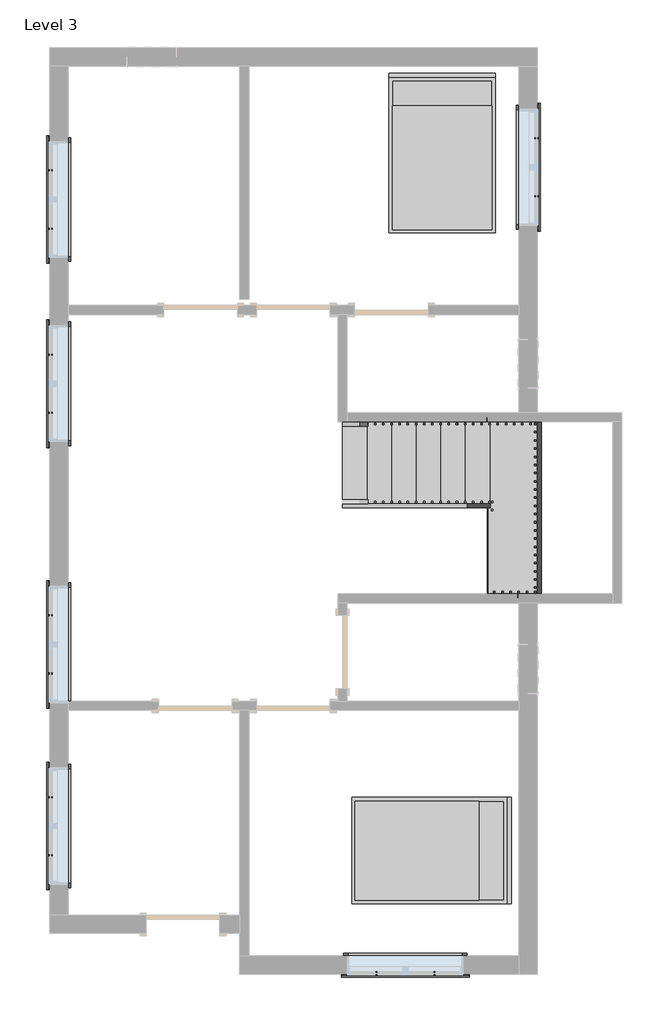
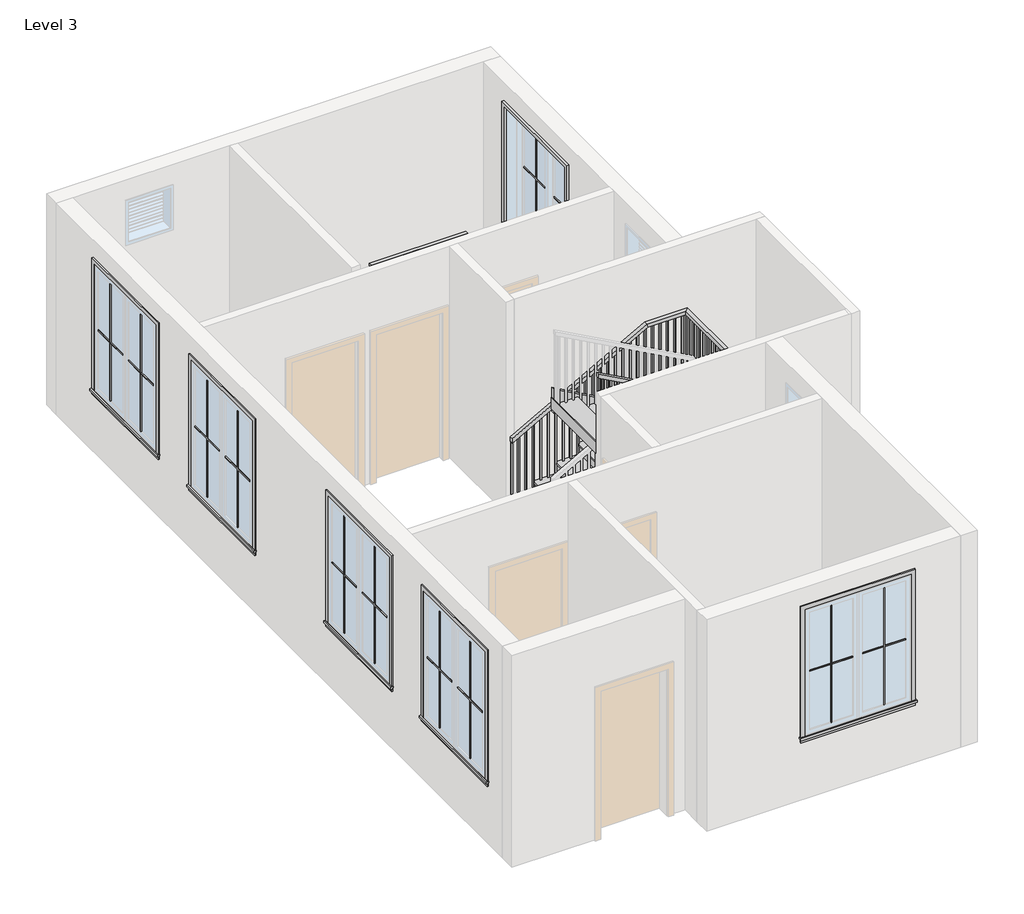
# One storey, part 2 of 2: 24 proxies, 5 members, 2 furniture elements, 1 railing, 1 stair flight.
"""IFC4 building model written with IfcOpenShell, lengths in millimetres."""

from ifc_helpers import new_model, si_unit, frame, origin, place, context, project, spatial, polyline, outline, extrude, faceted_brep, transform, mapped, element, save
from components import muntin_pattern_2x2_muntin_pattern_2x2_bff912c5, muntin_pattern_2x2_muntin_pattern_2x2_c2194282, trim_window_exterior_flat_with_sill_e04b3088, trim_window_interior_flat_picture_frame_2a7685fe, bed_17739_bed_17739_15c61121, stair_flight_656f6d92

model = new_model("IFC4")

# Units and contexts
model_context = context("Model", 3, world=origin())
ifc_project = project(units=[si_unit("LENGTHUNIT", "METRE", prefix="MILLI")], contexts=[model_context])

# Site, building, storey
site = spatial("IfcSite", under=ifc_project)
building = spatial("IfcBuilding", under=site)
storey = spatial("IfcBuildingStorey", under=building, Name="Level 3", Elevation=3200.4)

# Proxies
placement = place(None, origin())
muntin_pattern_2x2_muntin_pattern_2x2_shape = muntin_pattern_2x2_muntin_pattern_2x2_bff912c5(model_context)
element("IfcBuildingElementProxy", 1, Name="Muntin Pattern_2x2 : Muntin Pattern_2x2", ObjectType="Muntin Pattern_2x2 : Muntin Pattern_2x2", at=placement, inside=storey, context=model_context, shape_type="MappedRepresentation", body=[
    mapped(muntin_pattern_2x2_muntin_pattern_2x2_shape, transform((-4796.6888307, -4528.6107799, 4184.65), x_axis=(0.0, 1.0, 0.0), y_axis=(-1.0, 0.0, 0.0), z_axis=(0.0, 0.0, 1.0))),
])
element("IfcBuildingElementProxy", 2, Name="Muntin Pattern_2x2 : Muntin Pattern_2x2", ObjectType="Muntin Pattern_2x2 : Muntin Pattern_2x2", at=placement, inside=storey, context=model_context, shape_type="MappedRepresentation", body=[
    mapped(muntin_pattern_2x2_muntin_pattern_2x2_shape, transform((-4796.6888307, -2274.3607799, 4184.65), x_axis=(0.0, 1.0, 0.0), y_axis=(-1.0, 0.0, 0.0), z_axis=(0.0, 0.0, 1.0))),
])
element("IfcBuildingElementProxy", 3, Name="Muntin Pattern_2x2 : Muntin Pattern_2x2", ObjectType="Muntin Pattern_2x2 : Muntin Pattern_2x2", at=placement, inside=storey, context=model_context, shape_type="MappedRepresentation", body=[
    mapped(muntin_pattern_2x2_muntin_pattern_2x2_shape, transform((-26.2513307, -6000.2232799, 4184.65), x_axis=(-1.0, 0.0, 0.0), y_axis=(0.0, -1.0, 0.0), z_axis=(0.0, 0.0, 1.0))),
])
element("IfcBuildingElementProxy", 4, Name="Muntin Pattern_2x2 : Muntin Pattern_2x2", ObjectType="Muntin Pattern_2x2 : Muntin Pattern_2x2", at=placement, inside=storey, context=model_context, shape_type="MappedRepresentation", body=[
    mapped(muntin_pattern_2x2_muntin_pattern_2x2_shape, transform((1242.1611693, 4370.9142201, 4184.65), x_axis=(0.0, -1.0, 0.0), y_axis=(1.0, 0.0, 0.0), z_axis=(0.0, 0.0, 1.0))),
])
element("IfcBuildingElementProxy", 5, Name="Muntin Pattern_2x2 : Muntin Pattern_2x2", ObjectType="Muntin Pattern_2x2 : Muntin Pattern_2x2", at=placement, inside=storey, context=model_context, shape_type="MappedRepresentation", body=[
    mapped(muntin_pattern_2x2_muntin_pattern_2x2_shape, transform((-4796.6888307, 3250.1392201, 4184.65), x_axis=(0.0, 1.0, 0.0), y_axis=(-1.0, 0.0, 0.0), z_axis=(0.0, 0.0, 1.0))),
])
element("IfcBuildingElementProxy", 6, Name="Muntin Pattern_2x2 : Muntin Pattern_2x2", ObjectType="Muntin Pattern_2x2 : Muntin Pattern_2x2", at=placement, inside=storey, context=model_context, shape_type="MappedRepresentation", body=[
    mapped(muntin_pattern_2x2_muntin_pattern_2x2_shape, transform((-4796.6888307, 964.1392201, 4184.65), x_axis=(0.0, 1.0, 0.0), y_axis=(-1.0, 0.0, 0.0), z_axis=(0.0, 0.0, 1.0))),
])
muntin_pattern_2x2_muntin_pattern_2x2_2_shape = muntin_pattern_2x2_muntin_pattern_2x2_c2194282(model_context)
element("IfcBuildingElementProxy", 7, Name="Muntin Pattern_2x2 : Muntin Pattern_2x2", ObjectType="Muntin Pattern_2x2 : Muntin Pattern_2x2", at=placement, inside=storey, context=model_context, shape_type="MappedRepresentation", body=[
    mapped(muntin_pattern_2x2_muntin_pattern_2x2_2_shape, transform((-4796.6888307, -3807.8857799, 4184.65), x_axis=(0.0, -1.0, 0.0), y_axis=(1.0, 0.0, 0.0), z_axis=(0.0, 0.0, 1.0))),
])
element("IfcBuildingElementProxy", 8, Name="Muntin Pattern_2x2 : Muntin Pattern_2x2", ObjectType="Muntin Pattern_2x2 : Muntin Pattern_2x2", at=placement, inside=storey, context=model_context, shape_type="MappedRepresentation", body=[
    mapped(muntin_pattern_2x2_muntin_pattern_2x2_2_shape, transform((-4796.6888307, -1553.6357799, 4184.65), x_axis=(0.0, -1.0, 0.0), y_axis=(1.0, 0.0, 0.0), z_axis=(0.0, 0.0, 1.0))),
])
element("IfcBuildingElementProxy", 9, Name="Muntin Pattern_2x2 : Muntin Pattern_2x2", ObjectType="Muntin Pattern_2x2 : Muntin Pattern_2x2", at=placement, inside=storey, context=model_context, shape_type="MappedRepresentation", body=[
    mapped(muntin_pattern_2x2_muntin_pattern_2x2_2_shape, transform((-746.9763307, -6000.2232799, 4184.65), x_axis=(1.0, 0.0, 0.0), y_axis=(0.0, 1.0, 0.0), z_axis=(0.0, 0.0, 1.0))),
])
element("IfcBuildingElementProxy", 10, Name="Muntin Pattern_2x2 : Muntin Pattern_2x2", ObjectType="Muntin Pattern_2x2 : Muntin Pattern_2x2", at=placement, inside=storey, context=model_context, shape_type="MappedRepresentation", body=[
    mapped(muntin_pattern_2x2_muntin_pattern_2x2_2_shape, transform((1242.1611693, 3650.1892201, 4184.65), x_axis=(0.0, 1.0, 0.0), y_axis=(-1.0, 0.0, 0.0), z_axis=(0.0, 0.0, 1.0))),
])
element("IfcBuildingElementProxy", 11, Name="Muntin Pattern_2x2 : Muntin Pattern_2x2", ObjectType="Muntin Pattern_2x2 : Muntin Pattern_2x2", at=placement, inside=storey, context=model_context, shape_type="MappedRepresentation", body=[
    mapped(muntin_pattern_2x2_muntin_pattern_2x2_2_shape, transform((-4796.6888307, 3970.8642201, 4184.65), x_axis=(0.0, -1.0, 0.0), y_axis=(1.0, 0.0, 0.0), z_axis=(0.0, 0.0, 1.0))),
])
element("IfcBuildingElementProxy", 12, Name="Muntin Pattern_2x2 : Muntin Pattern_2x2", ObjectType="Muntin Pattern_2x2 : Muntin Pattern_2x2", at=placement, inside=storey, context=model_context, shape_type="MappedRepresentation", body=[
    mapped(muntin_pattern_2x2_muntin_pattern_2x2_2_shape, transform((-4796.6888307, 1684.8642201, 4184.65), x_axis=(0.0, -1.0, 0.0), y_axis=(1.0, 0.0, 0.0), z_axis=(0.0, 0.0, 1.0))),
])
trim_window_exterior_flat_with_sill_shape = trim_window_exterior_flat_with_sill_e04b3088(model_context)
element("IfcBuildingElementProxy", 13, Name="Trim-Window-Exterior-Flat : with Sill", ObjectType="Trim-Window-Exterior-Flat : with Sill", at=placement, inside=storey, context=model_context, shape_type="MappedRepresentation", body=[
    mapped(trim_window_exterior_flat_with_sill_shape, transform((-4806.2138307, -4168.2482799, 5943.6), x_axis=(0.0, -1.0, 0.0), y_axis=(0.0, 0.0, 1.0), z_axis=(-1.0, 0.0, 0.0))),
])
element("IfcBuildingElementProxy", 14, Name="Trim-Window-Exterior-Flat : with Sill", ObjectType="Trim-Window-Exterior-Flat : with Sill", at=placement, inside=storey, context=model_context, shape_type="MappedRepresentation", body=[
    mapped(trim_window_exterior_flat_with_sill_shape, transform((-4806.2138307, -1913.9982799, 5943.6), x_axis=(0.0, -1.0, 0.0), y_axis=(0.0, 0.0, 1.0), z_axis=(-1.0, 0.0, 0.0))),
])
element("IfcBuildingElementProxy", 15, Name="Trim-Window-Exterior-Flat : with Sill", ObjectType="Trim-Window-Exterior-Flat : with Sill", at=placement, inside=storey, context=model_context, shape_type="MappedRepresentation", body=[
    mapped(trim_window_exterior_flat_with_sill_shape, transform((-386.6138307, -6009.7482799, 5943.6), x_axis=(1.0, 0.0, 0.0), y_axis=(0.0, 0.0, 1.0), z_axis=(0.0, -1.0, 0.0))),
])
element("IfcBuildingElementProxy", 16, Name="Trim-Window-Exterior-Flat : with Sill", ObjectType="Trim-Window-Exterior-Flat : with Sill", at=placement, inside=storey, context=model_context, shape_type="MappedRepresentation", body=[
    mapped(trim_window_exterior_flat_with_sill_shape, transform((1251.6861693, 4010.5517201, 5943.6), x_axis=(0.0, 1.0, 0.0), y_axis=(0.0, 0.0, 1.0), z_axis=(1.0, 0.0, 0.0))),
])
element("IfcBuildingElementProxy", 17, Name="Trim-Window-Exterior-Flat : with Sill", ObjectType="Trim-Window-Exterior-Flat : with Sill", at=placement, inside=storey, context=model_context, shape_type="MappedRepresentation", body=[
    mapped(trim_window_exterior_flat_with_sill_shape, transform((-4806.2138307, 3610.5017201, 5943.6), x_axis=(0.0, -1.0, 0.0), y_axis=(0.0, 0.0, 1.0), z_axis=(-1.0, 0.0, 0.0))),
])
element("IfcBuildingElementProxy", 18, Name="Trim-Window-Exterior-Flat : with Sill", ObjectType="Trim-Window-Exterior-Flat : with Sill", at=placement, inside=storey, context=model_context, shape_type="MappedRepresentation", body=[
    mapped(trim_window_exterior_flat_with_sill_shape, transform((-4806.2138307, 1324.5017201, 5943.6), x_axis=(0.0, -1.0, 0.0), y_axis=(0.0, 0.0, 1.0), z_axis=(-1.0, 0.0, 0.0))),
])
trim_window_interior_flat_picture_frame_shape = trim_window_interior_flat_picture_frame_2a7685fe(model_context)
element("IfcBuildingElementProxy", 19, Name="Trim-Window-Interior-Flat : Picture Frame", ObjectType="Trim-Window-Interior-Flat : Picture Frame", at=placement, inside=storey, context=model_context, shape_type="MappedRepresentation", body=[
    mapped(trim_window_interior_flat_picture_frame_shape, transform((-4577.6138307, -4168.2482799, 5943.6), x_axis=(0.0, 1.0, 0.0), y_axis=(0.0, 0.0, 1.0), z_axis=(1.0, 0.0, 0.0))),
])
element("IfcBuildingElementProxy", 20, Name="Trim-Window-Interior-Flat : Picture Frame", ObjectType="Trim-Window-Interior-Flat : Picture Frame", at=placement, inside=storey, context=model_context, shape_type="MappedRepresentation", body=[
    mapped(trim_window_interior_flat_picture_frame_shape, transform((-4577.6138307, -1913.9982799, 5943.6), x_axis=(0.0, 1.0, 0.0), y_axis=(0.0, 0.0, 1.0), z_axis=(1.0, 0.0, 0.0))),
])
element("IfcBuildingElementProxy", 21, Name="Trim-Window-Interior-Flat : Picture Frame", ObjectType="Trim-Window-Interior-Flat : Picture Frame", at=placement, inside=storey, context=model_context, shape_type="MappedRepresentation", body=[
    mapped(trim_window_interior_flat_picture_frame_shape, transform((-386.6138307, -5781.1482799, 5943.6), x_axis=(-1.0, 0.0, 0.0), y_axis=(0.0, 0.0, 1.0), z_axis=(0.0, 1.0, 0.0))),
])
element("IfcBuildingElementProxy", 22, Name="Trim-Window-Interior-Flat : Picture Frame", ObjectType="Trim-Window-Interior-Flat : Picture Frame", at=placement, inside=storey, context=model_context, shape_type="MappedRepresentation", body=[
    mapped(trim_window_interior_flat_picture_frame_shape, transform((1023.0861693, 4010.5517201, 5943.6), x_axis=(0.0, -1.0, 0.0), y_axis=(0.0, 0.0, 1.0), z_axis=(-1.0, 0.0, 0.0))),
])
element("IfcBuildingElementProxy", 23, Name="Trim-Window-Interior-Flat : Picture Frame", ObjectType="Trim-Window-Interior-Flat : Picture Frame", at=placement, inside=storey, context=model_context, shape_type="MappedRepresentation", body=[
    mapped(trim_window_interior_flat_picture_frame_shape, transform((-4577.6138307, 3610.5017201, 5943.6), x_axis=(0.0, 1.0, 0.0), y_axis=(0.0, 0.0, 1.0), z_axis=(1.0, 0.0, 0.0))),
])
element("IfcBuildingElementProxy", 24, Name="Trim-Window-Interior-Flat : Picture Frame", ObjectType="Trim-Window-Interior-Flat : Picture Frame", at=placement, inside=storey, context=model_context, shape_type="MappedRepresentation", body=[
    mapped(trim_window_interior_flat_picture_frame_shape, transform((-4577.6138307, 1324.5017201, 5943.6), x_axis=(0.0, 1.0, 0.0), y_axis=(0.0, 0.0, 1.0), z_axis=(1.0, 0.0, 0.0))),
])

# Furniture
bed_17739_bed_17739_shape = bed_17739_bed_17739_15c61121(model_context)
element("IfcFurniture", 25, ObjectType="Bed_17739 : Bed_17739", at=placement, inside=storey, context=model_context, shape_type="MappedRepresentation", body=[
    mapped(bed_17739_bed_17739_shape, transform((70.5861693, 4162.9517201, 3200.4), x_axis=(1.0, 0.0, 0.0), y_axis=(0.0, 1.0, 0.0), z_axis=(0.0, 0.0, 1.0))),
])
element("IfcFurniture", 26, ObjectType="Bed_17739 : Bed_17739", at=placement, inside=storey, context=model_context, shape_type="MappedRepresentation", body=[
    mapped(bed_17739_bed_17739_shape, transform((-81.8138307, -4473.0482799, 3200.4), x_axis=(0.0, -1.0, 0.0), y_axis=(1.0, 0.0, 0.0), z_axis=(0.0, 0.0, 1.0))),
])

# Members
element("IfcMember", 27, ObjectType="Stringer - 2\" Width", at=placement, inside=storey, context=model_context, shape_type="SweptSolid", body=[
    extrude(outline(polyline([(3404.470617, -1167.6638307), (3200.4, -1167.6638307), (3200.4, -907.3693279), (4399.8752762, 1251.6861693), (4461.9333333, 1251.6861693), (4461.9333333, 735.7690587), (3404.470617, -1167.6638307)])), frame((0.0, 848.2517201, 0.0), z_axis=(0.0, 1.0, 0.0), x_axis=(0.0, 0.0, 1.0)), (0.0, 0.0, 1.0), 50.8),
])
element("IfcMember", 28, ObjectType="Stringer - 2\" Width", at=placement, inside=storey, context=model_context, shape_type="SweptSolid", body=[
    extrude(outline(polyline([(1251.6861693, 899.0517201), (1302.4861693, 899.0517201), (1302.4861693, -1285.3482799), (1251.6861693, -1285.3482799), (1251.6861693, 899.0517201)])), frame((0.0, 0.0, 4157.1333333), z_axis=(0.0, 0.0, 1.0), x_axis=(1.0, 0.0, 0.0)), (0.0, 0.0, 1.0), 304.8),
])
element("IfcMember", 29, ObjectType="Stringer - 2\" Width", at=placement, inside=storey, context=model_context, shape_type="SweptSolid", body=[
    extrude(outline(polyline([(4157.1333333, 1302.4861693), (4240.5539503, 1302.4861693), (5623.4428392, -1186.7138307), (5274.7641651, -1186.7138307), (4157.1333333, 825.0216665), (4157.1333333, 1302.4861693)])), frame((0.0, -1336.1482799, 0.0), z_axis=(0.0, 1.0, 0.0), x_axis=(0.0, 0.0, 1.0)), (0.0, 0.0, 1.0), 50.8),
])
element("IfcMember", 30, ObjectType="Stringer - 2\" Width", at=placement, inside=storey, context=model_context, shape_type="SweptSolid", body=[
    extrude(outline(polyline([(3404.470617, -1167.6638307), (3200.4, -1167.6638307), (3200.4, -907.3693279), (4047.0974984, 616.6861693), (4395.7761726, 616.6861693), (3404.470617, -1167.6638307)])), frame((0.0, -218.5482799, 0.0), z_axis=(0.0, 1.0, 0.0), x_axis=(0.0, 0.0, 1.0)), (0.0, 0.0, 1.0), 50.8),
])
element("IfcMember", 31, ObjectType="Stringer - 2\" Width", at=placement, inside=storey, context=model_context, shape_type="SweptSolid", body=[
    extrude(outline(polyline([(4244.653054, 667.4861693), (4593.3317281, 667.4861693), (5623.4428392, -1186.7138307), (5274.7641651, -1186.7138307), (4244.653054, 667.4861693)])), frame((0.0, -218.5482799, 0.0), z_axis=(0.0, 1.0, 0.0), x_axis=(0.0, 0.0, 1.0)), (0.0, 0.0, 1.0), 50.8),
])

# Railing
element("IfcRailing", 32, ObjectType="Handrail - Rectangular", at=placement, inside=storey, context=model_context, shape_type="SolidModel", body=[
    faceted_brep([(-1167.6638307, 848.2517201, 4284.1333333), (-1167.6638307, 848.2517201, 4226.0675836), (-1167.6638307, 797.4517201, 4226.0675836), (-1167.6638307, 797.4517201, 4284.1333333), (667.4861693, 848.2517201, 5300.1333333), (680.6099298, 848.2517201, 5249.3333333), (680.6099298, 797.4517201, 5249.3333333), (667.4861693, 797.4517201, 5300.1333333), (1251.6861693, 848.2517201, 5300.1333333), (1251.6861693, 848.2517201, 5249.3333333), (1200.8861693, 797.4517201, 5249.3333333), (1200.8861693, 797.4517201, 5300.1333333), (1251.6861693, -1285.3482799, 5300.1333333), (1251.6861693, -1285.3482799, 5249.3333333), (1200.8861693, -1234.5482799, 5249.3333333), (1200.8861693, -1234.5482799, 5300.1333333), (976.5195026, -1285.3482799, 5300.1333333), (963.5139215, -1285.3482799, 5249.3333333), (963.5139215, -1234.5482799, 5249.3333333), (976.5195026, -1234.5482799, 5300.1333333), (-1186.7138307, -1285.3482799, 6485.4666667), (-1186.7138307, -1234.5482799, 6485.4666667), (-1186.7138307, -1234.5482799, 6427.5403208), (-1186.7138307, -1285.3482799, 6427.5403208)], [[[0, 1, 2, 3]], [[1, 0, 4, 5]], [[2, 1, 5, 6]], [[3, 2, 6, 7]], [[0, 3, 7, 4]], [[5, 4, 8, 9]], [[6, 5, 9, 10]], [[7, 6, 10, 11]], [[4, 7, 11, 8]], [[9, 8, 12, 13]], [[10, 9, 13, 14]], [[11, 10, 14, 15]], [[8, 11, 15, 12]], [[13, 12, 16, 17]], [[14, 13, 17, 18]], [[15, 14, 18, 19]], [[12, 15, 19, 16]], [[20, 21, 22, 23]], [[17, 16, 20, 23]], [[18, 17, 23, 22]], [[19, 18, 22, 21]], [[16, 19, 21, 20]]]),
    extrude(outline(polyline([(6391.0060742, -1120.0388307), (5401.7333333, -1120.0388307), (5401.7333333, -1100.9888307), (6380.5677181, -1100.9888307), (6391.0060742, -1120.0388307)])), frame((0.0, -1269.4732799, 0.0), z_axis=(0.0, 1.0, 0.0), x_axis=(0.0, 0.0, 1.0)), (0.0, 0.0, 1.0), 19.05),
    extrude(outline(polyline([(6335.3348414, -1018.4388307), (5401.7333333, -1018.4388307), (5401.7333333, -999.3888307), (6324.8964852, -999.3888307), (6335.3348414, -1018.4388307)])), frame((0.0, -1269.4732799, 0.0), z_axis=(0.0, 1.0, 0.0), x_axis=(0.0, 0.0, 1.0)), (0.0, 0.0, 1.0), 19.05),
    extrude(outline(polyline([(6279.6636085, -916.8388307), (5401.7333333, -916.8388307), (5401.7333333, -897.7888307), (6269.2252523, -897.7888307), (6279.6636085, -916.8388307)])), frame((0.0, -1269.4732799, 0.0), z_axis=(0.0, 1.0, 0.0), x_axis=(0.0, 0.0, 1.0)), (0.0, 0.0, 1.0), 19.05),
    extrude(outline(polyline([(6223.9923756, -815.2388307), (5232.4, -815.2388307), (5232.4, -796.1888307), (6213.5540195, -796.1888307), (6223.9923756, -815.2388307)])), frame((0.0, -1269.4732799, 0.0), z_axis=(0.0, 1.0, 0.0), x_axis=(0.0, 0.0, 1.0)), (0.0, 0.0, 1.0), 19.05),
    extrude(outline(polyline([(6168.3211427, -713.6388307), (5232.4, -713.6388307), (5232.4, -694.5888307), (6157.8827866, -694.5888307), (6168.3211427, -713.6388307)])), frame((0.0, -1269.4732799, 0.0), z_axis=(0.0, 1.0, 0.0), x_axis=(0.0, 0.0, 1.0)), (0.0, 0.0, 1.0), 19.05),
    extrude(outline(polyline([(6112.6499099, -612.0388307), (5232.4, -612.0388307), (5232.4, -592.9888307), (6102.2115537, -592.9888307), (6112.6499099, -612.0388307)])), frame((0.0, -1269.4732799, 0.0), z_axis=(0.0, 1.0, 0.0), x_axis=(0.0, 0.0, 1.0)), (0.0, 0.0, 1.0), 19.05),
    extrude(outline(polyline([(6056.978677, -510.4388307), (5063.0666667, -510.4388307), (5063.0666667, -491.3888307), (6046.5403208, -491.3888307), (6056.978677, -510.4388307)])), frame((0.0, -1269.4732799, 0.0), z_axis=(0.0, 1.0, 0.0), x_axis=(0.0, 0.0, 1.0)), (0.0, 0.0, 1.0), 19.05),
    extrude(outline(polyline([(6001.3074441, -408.8388307), (5063.0666667, -408.8388307), (5063.0666667, -389.7888307), (5990.8690879, -389.7888307), (6001.3074441, -408.8388307)])), frame((0.0, -1269.4732799, 0.0), z_axis=(0.0, 1.0, 0.0), x_axis=(0.0, 0.0, 1.0)), (0.0, 0.0, 1.0), 19.05),
    extrude(outline(polyline([(5945.6362112, -307.2388307), (5063.0666667, -307.2388307), (5063.0666667, -288.1888307), (5935.1978551, -288.1888307), (5945.6362112, -307.2388307)])), frame((0.0, -1269.4732799, 0.0), z_axis=(0.0, 1.0, 0.0), x_axis=(0.0, 0.0, 1.0)), (0.0, 0.0, 1.0), 19.05),
    extrude(outline(polyline([(5889.9649784, -205.6388307), (4893.7333333, -205.6388307), (4893.7333333, -186.5888307), (5879.5266222, -186.5888307), (5889.9649784, -205.6388307)])), frame((0.0, -1269.4732799, 0.0), z_axis=(0.0, 1.0, 0.0), x_axis=(0.0, 0.0, 1.0)), (0.0, 0.0, 1.0), 19.05),
    extrude(outline(polyline([(5834.2937455, -104.0388307), (4893.7333333, -104.0388307), (4893.7333333, -84.9888307), (5823.8553893, -84.9888307), (5834.2937455, -104.0388307)])), frame((0.0, -1269.4732799, 0.0), z_axis=(0.0, 1.0, 0.0), x_axis=(0.0, 0.0, 1.0)), (0.0, 0.0, 1.0), 19.05),
    extrude(outline(polyline([(5778.6225126, -2.4388307), (4893.7333333, -2.4388307), (4893.7333333, 16.6111693), (5768.1841564, 16.6111693), (5778.6225126, -2.4388307)])), frame((0.0, -1269.4732799, 0.0), z_axis=(0.0, 1.0, 0.0), x_axis=(0.0, 0.0, 1.0)), (0.0, 0.0, 1.0), 19.05),
    extrude(outline(polyline([(5722.9512797, 99.1611693), (4724.4, 99.1611693), (4724.4, 118.2111693), (5712.5129236, 118.2111693), (5722.9512797, 99.1611693)])), frame((0.0, -1269.4732799, 0.0), z_axis=(0.0, 1.0, 0.0), x_axis=(0.0, 0.0, 1.0)), (0.0, 0.0, 1.0), 19.05),
    extrude(outline(polyline([(5667.2800469, 200.7611693), (4724.4, 200.7611693), (4724.4, 219.8111693), (5656.8416907, 219.8111693), (5667.2800469, 200.7611693)])), frame((0.0, -1269.4732799, 0.0), z_axis=(0.0, 1.0, 0.0), x_axis=(0.0, 0.0, 1.0)), (0.0, 0.0, 1.0), 19.05),
    extrude(outline(polyline([(5611.608814, 302.3611693), (4724.4, 302.3611693), (4724.4, 321.4111693), (5601.1704578, 321.4111693), (5611.608814, 302.3611693)])), frame((0.0, -1269.4732799, 0.0), z_axis=(0.0, 1.0, 0.0), x_axis=(0.0, 0.0, 1.0)), (0.0, 0.0, 1.0), 19.05),
    extrude(outline(polyline([(5555.9375811, 403.9611693), (4555.0666667, 403.9611693), (4555.0666667, 423.0111693), (5545.4992249, 423.0111693), (5555.9375811, 403.9611693)])), frame((0.0, -1269.4732799, 0.0), z_axis=(0.0, 1.0, 0.0), x_axis=(0.0, 0.0, 1.0)), (0.0, 0.0, 1.0), 19.05),
    extrude(outline(polyline([(5500.2663482, 505.5611693), (4555.0666667, 505.5611693), (4555.0666667, 524.6111693), (5489.8279921, 524.6111693), (5500.2663482, 505.5611693)])), frame((0.0, -1269.4732799, 0.0), z_axis=(0.0, 1.0, 0.0), x_axis=(0.0, 0.0, 1.0)), (0.0, 0.0, 1.0), 19.05),
    extrude(outline(polyline([(5444.5951153, 607.1611693), (4555.0666667, 607.1611693), (4555.0666667, 626.2111693), (5434.1567592, 626.2111693), (5444.5951153, 607.1611693)])), frame((0.0, -1269.4732799, 0.0), z_axis=(0.0, 1.0, 0.0), x_axis=(0.0, 0.0, 1.0)), (0.0, 0.0, 1.0), 19.05),
    extrude(outline(polyline([(5388.9238825, 708.7611693), (4385.7333333, 708.7611693), (4385.7333333, 727.8111693), (5378.4855263, 727.8111693), (5388.9238825, 708.7611693)])), frame((0.0, -1269.4732799, 0.0), z_axis=(0.0, 1.0, 0.0), x_axis=(0.0, 0.0, 1.0)), (0.0, 0.0, 1.0), 19.05),
    extrude(outline(polyline([(5333.2526496, 810.3611693), (4385.7333333, 810.3611693), (4385.7333333, 829.4111693), (5322.8142934, 829.4111693), (5333.2526496, 810.3611693)])), frame((0.0, -1269.4732799, 0.0), z_axis=(0.0, 1.0, 0.0), x_axis=(0.0, 0.0, 1.0)), (0.0, 0.0, 1.0), 19.05),
    extrude(outline(polyline([(5277.5814167, 911.9611693), (4385.7333333, 911.9611693), (4385.7333333, 931.0111693), (5267.1430606, 931.0111693), (5277.5814167, 911.9611693)])), frame((0.0, -1269.4732799, 0.0), z_axis=(0.0, 1.0, 0.0), x_axis=(0.0, 0.0, 1.0)), (0.0, 0.0, 1.0), 19.05),
    extrude(outline(polyline([(1032.6111693, -1269.4732799), (1013.5611693, -1269.4732799), (1013.5611693, -1250.4232799), (1032.6111693, -1250.4232799), (1032.6111693, -1269.4732799)])), frame((0.0, 0.0, 4385.7333333), z_axis=(0.0, 0.0, 1.0), x_axis=(1.0, 0.0, 0.0)), (0.0, 0.0, 1.0), 863.6),
    extrude(outline(polyline([(1134.2111693, -1269.4732799), (1115.1611693, -1269.4732799), (1115.1611693, -1250.4232799), (1134.2111693, -1250.4232799), (1134.2111693, -1269.4732799)])), frame((0.0, 0.0, 4385.7333333), z_axis=(0.0, 0.0, 1.0), x_axis=(1.0, 0.0, 0.0)), (0.0, 0.0, 1.0), 863.6),
    extrude(outline(polyline([(1235.8111693, -1199.6232799), (1235.8111693, -1218.6732799), (1216.7611693, -1218.6732799), (1216.7611693, -1199.6232799), (1235.8111693, -1199.6232799)])), frame((0.0, 0.0, 4385.7333333), z_axis=(0.0, 0.0, 1.0), x_axis=(1.0, 0.0, 0.0)), (0.0, 0.0, 1.0), 863.6),
    extrude(outline(polyline([(1235.8111693, -1098.0232799), (1235.8111693, -1117.0732799), (1216.7611693, -1117.0732799), (1216.7611693, -1098.0232799), (1235.8111693, -1098.0232799)])), frame((0.0, 0.0, 4385.7333333), z_axis=(0.0, 0.0, 1.0), x_axis=(1.0, 0.0, 0.0)), (0.0, 0.0, 1.0), 863.6),
    extrude(outline(polyline([(1235.8111693, -996.4232799), (1235.8111693, -1015.4732799), (1216.7611693, -1015.4732799), (1216.7611693, -996.4232799), (1235.8111693, -996.4232799)])), frame((0.0, 0.0, 4385.7333333), z_axis=(0.0, 0.0, 1.0), x_axis=(1.0, 0.0, 0.0)), (0.0, 0.0, 1.0), 863.6),
    extrude(outline(polyline([(1235.8111693, -894.8232799), (1235.8111693, -913.8732799), (1216.7611693, -913.8732799), (1216.7611693, -894.8232799), (1235.8111693, -894.8232799)])), frame((0.0, 0.0, 4385.7333333), z_axis=(0.0, 0.0, 1.0), x_axis=(1.0, 0.0, 0.0)), (0.0, 0.0, 1.0), 863.6),
    extrude(outline(polyline([(1235.8111693, -793.2232799), (1235.8111693, -812.2732799), (1216.7611693, -812.2732799), (1216.7611693, -793.2232799), (1235.8111693, -793.2232799)])), frame((0.0, 0.0, 4385.7333333), z_axis=(0.0, 0.0, 1.0), x_axis=(1.0, 0.0, 0.0)), (0.0, 0.0, 1.0), 863.6),
    extrude(outline(polyline([(1235.8111693, -691.6232799), (1235.8111693, -710.6732799), (1216.7611693, -710.6732799), (1216.7611693, -691.6232799), (1235.8111693, -691.6232799)])), frame((0.0, 0.0, 4385.7333333), z_axis=(0.0, 0.0, 1.0), x_axis=(1.0, 0.0, 0.0)), (0.0, 0.0, 1.0), 863.6),
    extrude(outline(polyline([(1235.8111693, -590.0232799), (1235.8111693, -609.0732799), (1216.7611693, -609.0732799), (1216.7611693, -590.0232799), (1235.8111693, -590.0232799)])), frame((0.0, 0.0, 4385.7333333), z_axis=(0.0, 0.0, 1.0), x_axis=(1.0, 0.0, 0.0)), (0.0, 0.0, 1.0), 863.6),
    extrude(outline(polyline([(1235.8111693, -488.4232799), (1235.8111693, -507.4732799), (1216.7611693, -507.4732799), (1216.7611693, -488.4232799), (1235.8111693, -488.4232799)])), frame((0.0, 0.0, 4385.7333333), z_axis=(0.0, 0.0, 1.0), x_axis=(1.0, 0.0, 0.0)), (0.0, 0.0, 1.0), 863.6),
    extrude(outline(polyline([(1235.8111693, -386.8232799), (1235.8111693, -405.8732799), (1216.7611693, -405.8732799), (1216.7611693, -386.8232799), (1235.8111693, -386.8232799)])), frame((0.0, 0.0, 4385.7333333), z_axis=(0.0, 0.0, 1.0), x_axis=(1.0, 0.0, 0.0)), (0.0, 0.0, 1.0), 863.6),
    extrude(outline(polyline([(1235.8111693, -285.2232799), (1235.8111693, -304.2732799), (1216.7611693, -304.2732799), (1216.7611693, -285.2232799), (1235.8111693, -285.2232799)])), frame((0.0, 0.0, 4385.7333333), z_axis=(0.0, 0.0, 1.0), x_axis=(1.0, 0.0, 0.0)), (0.0, 0.0, 1.0), 863.6),
    extrude(outline(polyline([(1235.8111693, -183.6232799), (1235.8111693, -202.6732799), (1216.7611693, -202.6732799), (1216.7611693, -183.6232799), (1235.8111693, -183.6232799)])), frame((0.0, 0.0, 4385.7333333), z_axis=(0.0, 0.0, 1.0), x_axis=(1.0, 0.0, 0.0)), (0.0, 0.0, 1.0), 863.6),
    extrude(outline(polyline([(1235.8111693, -82.0232799), (1235.8111693, -101.0732799), (1216.7611693, -101.0732799), (1216.7611693, -82.0232799), (1235.8111693, -82.0232799)])), frame((0.0, 0.0, 4385.7333333), z_axis=(0.0, 0.0, 1.0), x_axis=(1.0, 0.0, 0.0)), (0.0, 0.0, 1.0), 863.6),
    extrude(outline(polyline([(1235.8111693, 19.5767201), (1235.8111693, 0.5267201), (1216.7611693, 0.5267201), (1216.7611693, 19.5767201), (1235.8111693, 19.5767201)])), frame((0.0, 0.0, 4385.7333333), z_axis=(0.0, 0.0, 1.0), x_axis=(1.0, 0.0, 0.0)), (0.0, 0.0, 1.0), 863.6),
    extrude(outline(polyline([(1235.8111693, 121.1767201), (1235.8111693, 102.1267201), (1216.7611693, 102.1267201), (1216.7611693, 121.1767201), (1235.8111693, 121.1767201)])), frame((0.0, 0.0, 4385.7333333), z_axis=(0.0, 0.0, 1.0), x_axis=(1.0, 0.0, 0.0)), (0.0, 0.0, 1.0), 863.6),
    extrude(outline(polyline([(1235.8111693, 222.7767201), (1235.8111693, 203.7267201), (1216.7611693, 203.7267201), (1216.7611693, 222.7767201), (1235.8111693, 222.7767201)])), frame((0.0, 0.0, 4385.7333333), z_axis=(0.0, 0.0, 1.0), x_axis=(1.0, 0.0, 0.0)), (0.0, 0.0, 1.0), 863.6),
    extrude(outline(polyline([(1235.8111693, 324.3767201), (1235.8111693, 305.3267201), (1216.7611693, 305.3267201), (1216.7611693, 324.3767201), (1235.8111693, 324.3767201)])), frame((0.0, 0.0, 4385.7333333), z_axis=(0.0, 0.0, 1.0), x_axis=(1.0, 0.0, 0.0)), (0.0, 0.0, 1.0), 863.6),
    extrude(outline(polyline([(1235.8111693, 425.9767201), (1235.8111693, 406.9267201), (1216.7611693, 406.9267201), (1216.7611693, 425.9767201), (1235.8111693, 425.9767201)])), frame((0.0, 0.0, 4385.7333333), z_axis=(0.0, 0.0, 1.0), x_axis=(1.0, 0.0, 0.0)), (0.0, 0.0, 1.0), 863.6),
    extrude(outline(polyline([(1235.8111693, 527.5767201), (1235.8111693, 508.5267201), (1216.7611693, 508.5267201), (1216.7611693, 527.5767201), (1235.8111693, 527.5767201)])), frame((0.0, 0.0, 4385.7333333), z_axis=(0.0, 0.0, 1.0), x_axis=(1.0, 0.0, 0.0)), (0.0, 0.0, 1.0), 863.6),
    extrude(outline(polyline([(1235.8111693, 629.1767201), (1235.8111693, 610.1267201), (1216.7611693, 610.1267201), (1216.7611693, 629.1767201), (1235.8111693, 629.1767201)])), frame((0.0, 0.0, 4385.7333333), z_axis=(0.0, 0.0, 1.0), x_axis=(1.0, 0.0, 0.0)), (0.0, 0.0, 1.0), 863.6),
    extrude(outline(polyline([(1235.8111693, 730.7767201), (1235.8111693, 711.7267201), (1216.7611693, 711.7267201), (1216.7611693, 730.7767201), (1235.8111693, 730.7767201)])), frame((0.0, 0.0, 4385.7333333), z_axis=(0.0, 0.0, 1.0), x_axis=(1.0, 0.0, 0.0)), (0.0, 0.0, 1.0), 863.6),
    extrude(outline(polyline([(1159.6111693, 832.3767201), (1178.6611693, 832.3767201), (1178.6611693, 813.3267201), (1159.6111693, 813.3267201), (1159.6111693, 832.3767201)])), frame((0.0, 0.0, 4385.7333333), z_axis=(0.0, 0.0, 1.0), x_axis=(1.0, 0.0, 0.0)), (0.0, 0.0, 1.0), 863.6),
    extrude(outline(polyline([(1058.0111693, 832.3767201), (1077.0611693, 832.3767201), (1077.0611693, 813.3267201), (1058.0111693, 813.3267201), (1058.0111693, 832.3767201)])), frame((0.0, 0.0, 4385.7333333), z_axis=(0.0, 0.0, 1.0), x_axis=(1.0, 0.0, 0.0)), (0.0, 0.0, 1.0), 863.6),
    extrude(outline(polyline([(956.4111693, 832.3767201), (975.4611693, 832.3767201), (975.4611693, 813.3267201), (956.4111693, 813.3267201), (956.4111693, 832.3767201)])), frame((0.0, 0.0, 4385.7333333), z_axis=(0.0, 0.0, 1.0), x_axis=(1.0, 0.0, 0.0)), (0.0, 0.0, 1.0), 863.6),
    extrude(outline(polyline([(854.8111693, 832.3767201), (873.8611693, 832.3767201), (873.8611693, 813.3267201), (854.8111693, 813.3267201), (854.8111693, 832.3767201)])), frame((0.0, 0.0, 4385.7333333), z_axis=(0.0, 0.0, 1.0), x_axis=(1.0, 0.0, 0.0)), (0.0, 0.0, 1.0), 863.6),
    extrude(outline(polyline([(753.2111693, 832.3767201), (772.2611693, 832.3767201), (772.2611693, 813.3267201), (753.2111693, 813.3267201), (753.2111693, 832.3767201)])), frame((0.0, 0.0, 4385.7333333), z_axis=(0.0, 0.0, 1.0), x_axis=(1.0, 0.0, 0.0)), (0.0, 0.0, 1.0), 863.6),
    extrude(outline(polyline([(5233.2786562, 651.6111693), (4216.4, 651.6111693), (4216.4, 670.6611693), (5243.825369, 670.6611693), (5233.2786562, 651.6111693)])), frame((0.0, 813.3267201, 0.0), z_axis=(0.0, 1.0, 0.0), x_axis=(0.0, 0.0, 1.0)), (0.0, 0.0, 1.0), 19.05),
    extrude(outline(polyline([(5177.0295213, 550.0111693), (4216.4, 550.0111693), (4216.4, 569.0611693), (5187.5762341, 569.0611693), (5177.0295213, 550.0111693)])), frame((0.0, 813.3267201, 0.0), z_axis=(0.0, 1.0, 0.0), x_axis=(0.0, 0.0, 1.0)), (0.0, 0.0, 1.0), 19.05),
    extrude(outline(polyline([(5120.7803863, 448.4111693), (4216.4, 448.4111693), (4216.4, 467.4611693), (5131.3270991, 467.4611693), (5120.7803863, 448.4111693)])), frame((0.0, 813.3267201, 0.0), z_axis=(0.0, 1.0, 0.0), x_axis=(0.0, 0.0, 1.0)), (0.0, 0.0, 1.0), 19.05),
    extrude(outline(polyline([(5064.5312514, 346.8111693), (4047.0666667, 346.8111693), (4047.0666667, 365.8611693), (5075.0779642, 365.8611693), (5064.5312514, 346.8111693)])), frame((0.0, 813.3267201, 0.0), z_axis=(0.0, 1.0, 0.0), x_axis=(0.0, 0.0, 1.0)), (0.0, 0.0, 1.0), 19.05),
    extrude(outline(polyline([(5008.2821164, 245.2111693), (4047.0666667, 245.2111693), (4047.0666667, 264.2611693), (5018.8288292, 264.2611693), (5008.2821164, 245.2111693)])), frame((0.0, 813.3267201, 0.0), z_axis=(0.0, 1.0, 0.0), x_axis=(0.0, 0.0, 1.0)), (0.0, 0.0, 1.0), 19.05),
    extrude(outline(polyline([(4952.0329815, 143.6111693), (4047.0666667, 143.6111693), (4047.0666667, 162.6611693), (4962.5796943, 162.6611693), (4952.0329815, 143.6111693)])), frame((0.0, 813.3267201, 0.0), z_axis=(0.0, 1.0, 0.0), x_axis=(0.0, 0.0, 1.0)), (0.0, 0.0, 1.0), 19.05),
    extrude(outline(polyline([(4895.7838465, 42.0111693), (3877.7333333, 42.0111693), (3877.7333333, 61.0611693), (4906.3305593, 61.0611693), (4895.7838465, 42.0111693)])), frame((0.0, 813.3267201, 0.0), z_axis=(0.0, 1.0, 0.0), x_axis=(0.0, 0.0, 1.0)), (0.0, 0.0, 1.0), 19.05),
    extrude(outline(polyline([(4839.5347116, -59.5888307), (3877.7333333, -59.5888307), (3877.7333333, -40.5388307), (4850.0814244, -40.5388307), (4839.5347116, -59.5888307)])), frame((0.0, 813.3267201, 0.0), z_axis=(0.0, 1.0, 0.0), x_axis=(0.0, 0.0, 1.0)), (0.0, 0.0, 1.0), 19.05),
    extrude(outline(polyline([(4783.2855766, -161.1888307), (3877.7333333, -161.1888307), (3877.7333333, -142.1388307), (4793.8322895, -142.1388307), (4783.2855766, -161.1888307)])), frame((0.0, 813.3267201, 0.0), z_axis=(0.0, 1.0, 0.0), x_axis=(0.0, 0.0, 1.0)), (0.0, 0.0, 1.0), 19.05),
    extrude(outline(polyline([(4727.0364417, -262.7888307), (3708.4, -262.7888307), (3708.4, -243.7388307), (4737.5831545, -243.7388307), (4727.0364417, -262.7888307)])), frame((0.0, 813.3267201, 0.0), z_axis=(0.0, 1.0, 0.0), x_axis=(0.0, 0.0, 1.0)), (0.0, 0.0, 1.0), 19.05),
    extrude(outline(polyline([(4670.7873068, -364.3888307), (3708.4, -364.3888307), (3708.4, -345.3388307), (4681.3340196, -345.3388307), (4670.7873068, -364.3888307)])), frame((0.0, 813.3267201, 0.0), z_axis=(0.0, 1.0, 0.0), x_axis=(0.0, 0.0, 1.0)), (0.0, 0.0, 1.0), 19.05),
    extrude(outline(polyline([(4614.5381718, -465.9888307), (3708.4, -465.9888307), (3708.4, -446.9388307), (4625.0848846, -446.9388307), (4614.5381718, -465.9888307)])), frame((0.0, 813.3267201, 0.0), z_axis=(0.0, 1.0, 0.0), x_axis=(0.0, 0.0, 1.0)), (0.0, 0.0, 1.0), 19.05),
    extrude(outline(polyline([(4558.2890369, -567.5888307), (3539.0666667, -567.5888307), (3539.0666667, -548.5388307), (4568.8357497, -548.5388307), (4558.2890369, -567.5888307)])), frame((0.0, 813.3267201, 0.0), z_axis=(0.0, 1.0, 0.0), x_axis=(0.0, 0.0, 1.0)), (0.0, 0.0, 1.0), 19.05),
    extrude(outline(polyline([(4502.0399019, -669.1888307), (3539.0666667, -669.1888307), (3539.0666667, -650.1388307), (4512.5866147, -650.1388307), (4502.0399019, -669.1888307)])), frame((0.0, 813.3267201, 0.0), z_axis=(0.0, 1.0, 0.0), x_axis=(0.0, 0.0, 1.0)), (0.0, 0.0, 1.0), 19.05),
    extrude(outline(polyline([(4445.790767, -770.7888307), (3539.0666667, -770.7888307), (3539.0666667, -751.7388307), (4456.3374798, -751.7388307), (4445.790767, -770.7888307)])), frame((0.0, 813.3267201, 0.0), z_axis=(0.0, 1.0, 0.0), x_axis=(0.0, 0.0, 1.0)), (0.0, 0.0, 1.0), 19.05),
    extrude(outline(polyline([(4389.541632, -872.3888307), (3369.7333333, -872.3888307), (3369.7333333, -853.3388307), (4400.0883448, -853.3388307), (4389.541632, -872.3888307)])), frame((0.0, 813.3267201, 0.0), z_axis=(0.0, 1.0, 0.0), x_axis=(0.0, 0.0, 1.0)), (0.0, 0.0, 1.0), 19.05),
    extrude(outline(polyline([(4333.2924971, -973.9888307), (3369.7333333, -973.9888307), (3369.7333333, -954.9388307), (4343.8392099, -954.9388307), (4333.2924971, -973.9888307)])), frame((0.0, 813.3267201, 0.0), z_axis=(0.0, 1.0, 0.0), x_axis=(0.0, 0.0, 1.0)), (0.0, 0.0, 1.0), 19.05),
    extrude(outline(polyline([(4277.0433621, -1075.5888307), (3369.7333333, -1075.5888307), (3369.7333333, -1056.5388307), (4287.5900749, -1056.5388307), (4277.0433621, -1075.5888307)])), frame((0.0, 813.3267201, 0.0), z_axis=(0.0, 1.0, 0.0), x_axis=(0.0, 0.0, 1.0)), (0.0, 0.0, 1.0), 19.05),
    extrude(outline(polyline([(1235.8111693, -1250.4232799), (1235.8111693, -1269.4732799), (1216.7611693, -1269.4732799), (1216.7611693, -1250.4232799), (1235.8111693, -1250.4232799)])), frame((0.0, 0.0, 4385.7333333), z_axis=(0.0, 0.0, 1.0), x_axis=(1.0, 0.0, 0.0)), (0.0, 0.0, 1.0), 863.6),
    extrude(outline(polyline([(1216.7611693, 832.3767201), (1235.8111693, 832.3767201), (1235.8111693, 813.3267201), (1216.7611693, 813.3267201), (1216.7611693, 832.3767201)])), frame((0.0, 0.0, 4385.7333333), z_axis=(0.0, 0.0, 1.0), x_axis=(1.0, 0.0, 0.0)), (0.0, 0.0, 1.0), 863.6),
    extrude(outline(polyline([(6427.5403208, -1186.7138307), (5401.7333333, -1186.7138307), (5401.7333333, -1167.6638307), (6417.1019647, -1167.6638307), (6427.5403208, -1186.7138307)])), frame((0.0, -1269.4732799, 0.0), z_axis=(0.0, 1.0, 0.0), x_axis=(0.0, 0.0, 1.0)), (0.0, 0.0, 1.0), 19.05),
    extrude(outline(polyline([(4226.0675836, -1167.6638307), (3369.7333333, -1167.6638307), (3369.7333333, -1148.6138307), (4236.6142964, -1148.6138307), (4226.0675836, -1167.6638307)])), frame((0.0, 813.3267201, 0.0), z_axis=(0.0, 1.0, 0.0), x_axis=(0.0, 0.0, 1.0)), (0.0, 0.0, 1.0), 19.05),
])

# Stair flight
stair_flight_shape = stair_flight_656f6d92(model_context)
element("IfcStairFlight", 33, ObjectType="2\" Tread 1\" Nosing 1/4\" Riser", at=placement, inside=storey, context=model_context, shape_type="MappedRepresentation", body=[
    mapped(stair_flight_shape, transform((0.0, 0.0, 0.0), x_axis=(1.0, 0.0, 0.0), y_axis=(0.0, 1.0, 0.0), z_axis=(0.0, 0.0, 1.0))),
])

save(model, "model.ifc")

# Revit data of these elements
# Type "Muntin Pattern_2x2 : Muntin Pattern_2x2"
#   Width [instance default] = 4' - 0"
#   Thickness = 0' - 0 1/2"
#   Height [instance default] = 4' - 0"
#   Distance = 0' - 0 3/4"
#   Interior Material [instance default] = none
#   Exterior Material [instance default] = none
#   Default Elevation = 0
# Type "Trim-Window-Exterior-Flat : with Sill"
#   Trim Width = 0' - 2 1/4"
#   Trim Thickness_Picture Frame = 0' - 1 1/4"
#   Trim Thickness_with Sill = 0' - 0 3/4"
#   Sill Thickness = 0' - 1 1/4"
#   Opening Width [instance default] = 2' - 0"
#   Opening Height [instance default] = 3' - 0"
#   Default Elevation = 4' - 0"
#   Sill = yes
#   Picture Frame = no
#   Trim Material [instance default] = none
# Type "Trim-Window-Interior-Flat : Picture Frame"
#   Trim Thickness_Picture Frame = 0' - 1 1/4"
#   Trim Width = 0' - 2 1/4"
#   Trim Thickness_with Sill = 0' - 0 3/4"
#   Sill Thickness = 0' - 1 1/4"
#   Opening Width [instance default] = 2' - 0"
#   Opening Height [instance default] = 3' - 0"
#   Default Elevation = 4' - 0"
#   Sill = no
#   Picture Frame = yes
#   Trim Material [instance default] = none
# Type "Bed_17739 : Bed_17739"
#   Default Elevation = 0
# Type "Handrail - Rectangular"
#   Assembly Code = "C2010400"
#   built-in parameter 1008612 = 0.0416667 (stored number, unit not read)
#   built-in parameter 1008611 = 0.0416667 (stored number, unit not read)
#   built-in parameter 1008609 = 0.333333 (stored number, unit not read)
#   built-in parameter 1008604 = 0.166667 (stored number, unit not read)
#   built-in parameter 1008603 = 0.166667 (stored number, unit not read)
#   Railing Height = 3' - 0"
#   built-in parameter 1008630 = 2
#   built-in parameter 1008610 = 2
#   built-in parameter 1008618 = Baluster - Square : 3/4"
# Elements 1, 2, 3, 4, 5, 6, 7, 8, 9, 10, 11, 12 (IfcBuildingElementProxy, "Muntin Pattern_2x2 : Muntin Pattern_2x2")
#   Width = 1' - 11 1/8"
#   Height = 5' - 6 1/2"
#   Interior Material = Wood - Stained
#   Exterior Material = Clad - White
#   Phase Created = New Construction
#   Materials on its faces: "Clad - White", "Wood - Stained"
# Elements 13, 14, 15, 16, 17, 18 (IfcBuildingElementProxy, "Trim-Window-Exterior-Flat : with Sill")
#   Opening Width = 4' - 9"
#   Opening Height = 6' - 0"
#   Trim Material = Clad - White
#   Phase Created = New Construction
#   Materials on its faces: "Clad - White"
# Elements 19, 20, 21, 22, 23, 24 (IfcBuildingElementProxy, "Trim-Window-Interior-Flat : Picture Frame")
#   Opening Width = 4' - 9"
#   Opening Height = 6' - 0"
#   Trim Material = Wood - Stained
#   Phase Created = New Construction
#   Materials on its faces: "Wood - Stained"
# Elements 25, 26 (IfcFurniture, "Bed_17739 : Bed_17739")
#   Phase Created = New Construction
#   Materials on its faces: "legs", "sheets", "bed frame", "Blanket"
# Elements 27, 28, 29, 30, 31 (IfcMember, "Stringer - 2\" Width")
#   Phase Created = New Construction
# Element 32 (IfcRailing, "Handrail - Rectangular")
#   Phase Created = New Construction
# Element 33 (IfcStairFlight, "2\" Tread 1\" Nosing 1/4\" Riser")
#   Phase Created = New Construction
# Materials
#   "Clad - White": class "Wood", colour RGB 242 242 238, transparency 0, Cost = 0
#   "Wood - Stained": class "Wood", colour RGB 224 178 126, transparency 0, Cost = 0
#   "legs": colour RGB 90 73 37, transparency 0, Cost = 0
#   "sheets": colour RGB 200 195 176, transparency 0, Cost = 0
#   "bed frame": colour RGB 90 73 37, transparency 0, Cost = 0
#   "Blanket": class "System", colour RGB 59 0 1, transparency 0, Cost = 0
